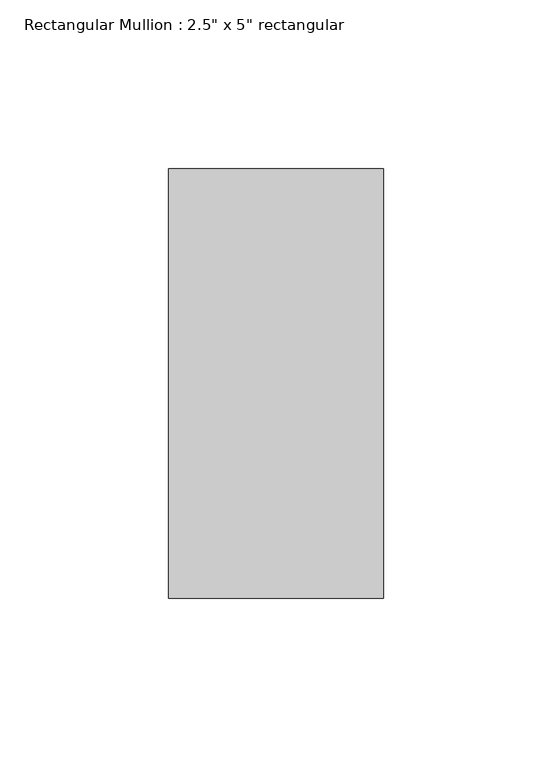
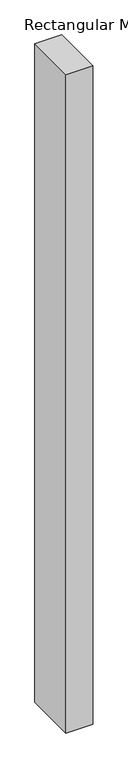
"""IFC4 building model written with IfcOpenShell, lengths in millimetres: member geometry."""

from ifc_helpers import new_model, si_unit, frame, origin, place, context, project, spatial, polyline, outline, extrude, source, transform, mapped, element, save


def member_f18c796a(model_context):
    return source(origin(), model_context, "Body", "SweptSolid", [
        extrude(outline(polyline([(0.0, 63.5), (0.0, -63.5), (-63.5, -63.5), (-63.5, 63.5), (0.0, 63.5)])), frame((0.0, 0.0, -1646.9365008), z_axis=(0.0, 0.0, 1.0), x_axis=(1.0, 0.0, 0.0)), (0.0, 0.0, 1.0), 1646.9365008),
    ])


if __name__ == "__main__":
    model = new_model("IFC4")
    model_context = context("Model", 3, world=origin())
    ifc_project = project(units=[si_unit("LENGTHUNIT", "METRE", prefix="MILLI")], contexts=[model_context])
    site = spatial("IfcSite", under=ifc_project)
    building = spatial("IfcBuilding", under=site)
    placement = place(None, origin())
    member_shape = member_f18c796a(model_context)
    element("IfcMember", 1, ObjectType="Rectangular Mullion : 2.5\" x 5\" rectangular", at=placement, inside=building, context=model_context, shape_type="MappedRepresentation", body=[
        mapped(member_shape, transform((0.0, 0.0, 0.0), x_axis=(1.0, 0.0, 0.0), y_axis=(0.0, 1.0, 0.0), z_axis=(0.0, 0.0, 1.0))),
    ])
    save(model, "model.ifc")

# Revit data of these elements
# Type "Rectangular Mullion : 2.5\" x 5\" rectangular"
#   built-in parameter 1007304 = 0.416667 (stored number, unit not read)
#   built-in parameter 1007301 = 0.104167 (stored number, unit not read)
#   built-in parameter 1007300 = 0.104167 (stored number, unit not read)
# Element 1 (IfcMember, "Rectangular Mullion : 2.5\" x 5\" rectangular")
#   Materials on its faces: "Aluminum"
# Materials
#   "Aluminum": class "Metal", colour RGB 247 247 247, transparency 0, Description = "Aluminum 6061", Cost = 0
